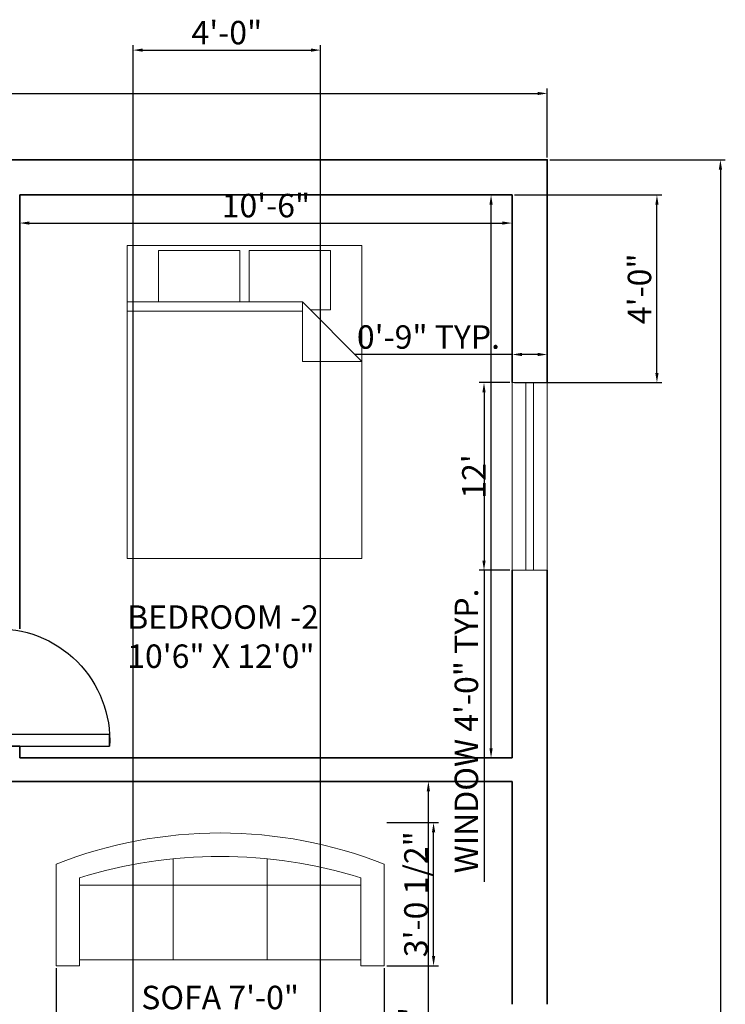
# Model space of a CAD drawing. Units: inches. Extents: x 2117 to 2588, y 1610 to 2201.
# Tile 4 of 4: x 2407 to 2588, y 1920 to 2172. Entities that reach past the tile are written whole.
import ezdxf

# ---------------------------------------------------------------- set-up
doc = ezdxf.new("R2010")
doc.units = ezdxf.units.IN
for name, color, linetype, lineweight in [('A-ANNO-DIMS', 2, 'Continuous', 18), ('A-AREA-IDEN', 7, 'Continuous', 25), ('A-DOOR', 4, 'Continuous', 25), ('A-FURN', 8, 'Continuous', 18), ('A-WALL', 7, 'Continuous', 35), ('WINDOW', 150, 'Continuous', 18)]:
    doc.layers.add(name, color=color, linetype=linetype, lineweight=lineweight)
doc.styles.get("Standard").update_dxf_attribs({"font": 'arial.ttf'})
doc.dimstyles.new('ISO-25', dxfattribs={"dimtxt": 6, "dimasz": 2.5, "dimexe": 1.25, "dimexo": 0.625, "dimtad": 1, "dimlunit": 3, "dimtxsty": 'Standard', "dimcen": 2.5, "dimadec": 0, "dimazin": 0, "dimtfac": 1, "dimtmove": 0, "dimatfit": 3, "dimfxl": 1, "dimarcsym": 0})

# ---------------------------------------------------------------- blocks, each defined once
blk = doc.blocks.new('*D1')
at = {"layer": 'A-ANNO-DIMS', "color": 0, "lineweight": -2, "transparency": 16777216}
for p, q in [((2407.08, 2126.4), (2407.08, 2118.59)), ((2533.08, 2126.4), (2533.08, 2118.59)), ((2409.58, 2119.84), (2530.58, 2119.84))]:
    blk.add_line(p, q, dxfattribs=at)
at = {"layer": 'A-ANNO-DIMS', "color": 0, "transparency": 16777216}
for points in [[(2409.58, 2120.26), (2409.58, 2119.43), (2407.08, 2119.84)], [(2530.58, 2120.26), (2530.58, 2119.43), (2533.08, 2119.84)]]:
    blk.add_solid(points, dxfattribs=at)
at = {"layer": 'Defpoints', "color": 0, "transparency": 16777216}
for p in [(2407.08, 2127.03), (2533.08, 2127.03), (2533.08, 2119.84)]:
    blk.add_point(p, dxfattribs=at)
at = {"layer": 'A-ANNO-DIMS', "color": 0, "transparency": 16777216, "insert": (2470.08, 2123.53), "char_height": 6, "attachment_point": 5}
blk.add_mtext('10\'-6"', dxfattribs=at)
blk = doc.blocks.new('*D2')
at = {"layer": 'A-ANNO-DIMS', "color": 0, "lineweight": -2, "transparency": 16777216}
for p, q in [((2532.45, 2127.03), (2526.43, 2127.03)), ((2527.68, 1985.53), (2527.68, 2124.53)), ((2532.45, 1983.03), (2526.43, 1983.03))]:
    blk.add_line(p, q, dxfattribs=at)
at = {"layer": 'A-ANNO-DIMS', "color": 0, "transparency": 16777216}
for points in [[(2527.27, 2124.53), (2528.1, 2124.53), (2527.68, 2127.03)], [(2527.27, 1985.53), (2528.1, 1985.53), (2527.68, 1983.03)]]:
    blk.add_solid(points, dxfattribs=at)
at = {"layer": 'Defpoints', "color": 0, "transparency": 16777216}
for p in [(2527.68, 2127.03), (2533.08, 2127.03), (2533.08, 1983.03)]:
    blk.add_point(p, dxfattribs=at)
at = {"layer": 'A-ANNO-DIMS', "color": 0, "transparency": 16777216, "insert": (2524.05, 2055.03), "char_height": 6, "attachment_point": 5, "rotation": 90}
blk.add_mtext("12'", dxfattribs=at)
blk = doc.blocks.new('*D16')
at = {"layer": 'A-ANNO-DIMS', "color": 0, "lineweight": -2, "transparency": 16777216}
for p, q in [((2532.45, 1977.03), (2510.4, 1977.03)), ((2511.65, 1841.53), (2511.65, 1974.53)), ((2532.45, 1839.03), (2510.4, 1839.03))]:
    blk.add_line(p, q, dxfattribs=at)
at = {"layer": 'A-ANNO-DIMS', "color": 0, "transparency": 16777216}
for points in [[(2511.23, 1974.53), (2512.06, 1974.53), (2511.65, 1977.03)], [(2511.23, 1841.53), (2512.06, 1841.53), (2511.65, 1839.03)]]:
    blk.add_solid(points, dxfattribs=at)
at = {"layer": 'Defpoints', "color": 0, "transparency": 16777216}
for p in [(2511.65, 1977.03), (2533.08, 1977.03), (2533.08, 1839.03)]:
    blk.add_point(p, dxfattribs=at)
at = {"layer": 'A-ANNO-DIMS', "color": 0, "transparency": 16777216, "insert": (2507.96, 1908.03), "char_height": 6, "attachment_point": 5, "rotation": 90}
blk.add_mtext('11\'-6"', dxfattribs=at)
blk = doc.blocks.new('Sofa - Roundback 7 ft.')
for p, q in [((-12.00002, -32.4421), (-12.00003, -6.5971)), ((11.99997, -32.4421), (11.99998, -6.5971)), ((-36.000027, -34), (-36.000027, -11.4696)), ((35.99998, -34), (35.99998, -11.4696)), ((-35.999844, -13.3819), (35.9998, -13.3819)), ((-36.000027, -32.4421), (35.99998, -32.4421))]:
    blk.add_line(p, q)
for points in [[(-36.000027, -34), (-42.000027, -34), (-42.000027, -8)], [(41.99998, -8), (41.99998, -34), (35.99998, -34)]]:
    blk.add_lwpolyline(points)
for centre, radius, start, end in [((0, -114.25), 114.25, 68.43141, 111.5686), ((-0.00001, -127.1968), 121.1968, 72.72033, 107.2797)]:
    blk.add_arc(centre, radius, start, end)
blk = doc.blocks.new('Bed - Queen')
for p, q in [((0, -80.00003), (0, 0)), ((0, 0), (59.99999, 0)), ((59.99999, 0), (59.99999, -80.00003)), ((7.99999, -1.2), (28.79998, -1.2)), ((7.99999, -14.4), (7.99999, -1.2)), ((28.79998, -1.2), (28.79998, -14.4)), ((31.19999, -1.2), (51.99999, -1.2)), ((31.19999, -14.4), (31.19999, -1.2)), ((51.99999, -1.2), (51.99999, -16.4)), ((0, -14.4), (44.8, -14.4)), ((59.99999, -29.6), (44.8, -14.4)), ((44.8, -14.4), (44.8, -29.6)), ((44.8, -16.8), (0, -16.8)), ((51.99999, -16.4), (46.79936, -16.4)), ((44.8, -29.6), (59.99999, -29.6)), ((59.99999, -80.00003), (0, -80.00003))]:
    blk.add_line(p, q)
blk = doc.blocks.new('*D30')
at = {"layer": 'A-ANNO-DIMS', "color": 0, "lineweight": -2, "transparency": 16777216}
for p, q in [((2158.08, 2136.65), (2158.08, 2154.24)), ((2542.08, 2136.65), (2542.08, 2154.24)), ((2160.58, 2152.99), (2539.58, 2152.99))]:
    blk.add_line(p, q, dxfattribs=at)
at = {"layer": 'A-ANNO-DIMS', "color": 0, "transparency": 16777216}
for points in [[(2160.58, 2153.4), (2160.58, 2152.57), (2158.08, 2152.99)], [(2539.58, 2153.4), (2539.58, 2152.57), (2542.08, 2152.99)]]:
    blk.add_solid(points, dxfattribs=at)
at = {"layer": 'Defpoints', "color": 0, "transparency": 16777216}
for p in [(2542.08, 2152.99), (2158.08, 2136.03), (2542.08, 2136.03)]:
    blk.add_point(p, dxfattribs=at)
at = {"layer": 'A-ANNO-DIMS', "color": 0, "transparency": 16777216, "insert": (2350.08, 2156.68), "char_height": 6, "attachment_point": 5}
blk.add_mtext("32'", dxfattribs=at)
blk = doc.blocks.new('*D31')
at = {"layer": 'A-ANNO-DIMS', "color": 0, "lineweight": -2, "transparency": 16777216}
for p, q in [((2542.7, 2136.03), (2587.62, 2136.03)), ((2586.37, 2133.53), (2586.37, 1658.53)), ((2542.7, 1656.03), (2587.62, 1656.03))]:
    blk.add_line(p, q, dxfattribs=at)
at = {"layer": 'A-ANNO-DIMS', "color": 0, "transparency": 16777216}
for points in [[(2585.96, 2133.53), (2586.79, 2133.53), (2586.37, 2136.03)], [(2585.96, 1658.53), (2586.79, 1658.53), (2586.37, 1656.03)]]:
    blk.add_solid(points, dxfattribs=at)
at = {"layer": 'Defpoints', "color": 0, "transparency": 16777216}
for p in [(2542.08, 2136.03), (2542.08, 1656.03), (2586.37, 1656.03)]:
    blk.add_point(p, dxfattribs=at)
at = {"layer": 'A-ANNO-DIMS', "color": 0, "transparency": 16777216, "insert": (2582.68, 1896.03), "char_height": 6, "attachment_point": 5, "rotation": 90}
blk.add_mtext("40'", dxfattribs=at)
blk = doc.blocks.new('WIN-48IN-9IN-WALL')
for p, q in [((9, 48), (0, 48)), ((0, 0), (0, 48)), ((3.5, 0), (3.5, 48)), ((5.5, 0), (5.5, 48)), ((9, 0), (9, 48)), ((9, 0), (0, 0))]:
    blk.add_line(p, q)
blk = doc.blocks.new('DOOR-SWING-30IN')
blk.add_lwpolyline([(30.04, 0), (0.04, 0), (0.04, 3), (30.04, 3)], close=True)
blk.add_arc((28.54, 1.5), 28.54, 86.9872, 183.0128)
blk = doc.blocks.new('*D37')
at = {"layer": 'A-ANNO-DIMS', "color": 0, "lineweight": -2, "transparency": 16777216}
for p, q in [((2532.45, 2079.03), (2524.63, 2079.03)), ((2525.88, 2076.53), (2525.88, 2033.53)), ((2532.45, 2031.03), (2524.63, 2031.03)), ((2525.88, 2031.03), (2525.88, 1951.35))]:
    blk.add_line(p, q, dxfattribs=at)
at = {"layer": 'A-ANNO-DIMS', "color": 0, "transparency": 16777216}
for points in [[(2525.46, 2076.53), (2526.29, 2076.53), (2525.88, 2079.03)], [(2525.46, 2033.53), (2526.29, 2033.53), (2525.88, 2031.03)]]:
    blk.add_solid(points, dxfattribs=at)
at = {"layer": 'Defpoints', "color": 0, "transparency": 16777216}
for p in [(2533.08, 2079.03), (2525.88, 2031.03), (2533.08, 2031.03)]:
    blk.add_point(p, dxfattribs=at)
at = {"layer": 'A-ANNO-DIMS', "color": 0, "transparency": 16777216, "insert": (2522.15, 1989.94), "char_height": 6, "attachment_point": 5, "rotation": 90}
blk.add_mtext('WINDOW 4\'-0" TYP.', dxfattribs=at)
blk = doc.blocks.new('*D38')
at = {"layer": 'A-ANNO-DIMS', "color": 0, "lineweight": -2, "transparency": 16777216}
for p, q in [((2533.08, 2086.23), (2492.75, 2086.23)), ((2533.08, 2079.65), (2533.08, 2087.48)), ((2539.58, 2086.23), (2535.58, 2086.23)), ((2542.08, 2079.65), (2542.08, 2087.48))]:
    blk.add_line(p, q, dxfattribs=at)
at = {"layer": 'A-ANNO-DIMS', "color": 0, "transparency": 16777216}
for points in [[(2535.58, 2086.65), (2535.58, 2085.81), (2533.08, 2086.23)], [(2539.58, 2086.65), (2539.58, 2085.81), (2542.08, 2086.23)]]:
    blk.add_solid(points, dxfattribs=at)
at = {"layer": 'Defpoints', "color": 0, "transparency": 16777216}
for p in [(2533.08, 2086.23), (2533.08, 2079.03), (2542.08, 2079.03)]:
    blk.add_point(p, dxfattribs=at)
at = {"layer": 'A-ANNO-DIMS', "color": 0, "transparency": 16777216, "insert": (2511.66, 2089.92), "char_height": 6, "attachment_point": 5}
blk.add_mtext('0\'-9" TYP.', dxfattribs=at)
blk = doc.blocks.new('*D47')
at = {"layer": 'A-ANNO-DIMS', "color": 0, "lineweight": -2, "transparency": 16777216}
for p, q in [((2403.45, 2120.46), (2403.45, 2156.7)), ((2399.12, 2120.46), (2404.7, 2120.46)), ((2403.45, 2089.91), (2403.45, 2117.96)), ((2399.12, 2087.41), (2404.7, 2087.41))]:
    blk.add_line(p, q, dxfattribs=at)
at = {"layer": 'A-ANNO-DIMS', "color": 0, "transparency": 16777216}
for points in [[(2403.04, 2117.96), (2403.87, 2117.96), (2403.45, 2120.46)], [(2403.04, 2089.91), (2403.87, 2089.91), (2403.45, 2087.41)]]:
    blk.add_solid(points, dxfattribs=at)
at = {"layer": 'Defpoints', "color": 0, "transparency": 16777216}
for p in [(2398.5, 2120.46), (2403.45, 2120.46), (2398.5, 2087.41)]:
    blk.add_point(p, dxfattribs=at)
at = {"layer": 'A-ANNO-DIMS', "color": 0, "transparency": 16777216, "insert": (2399.73, 2139.83), "char_height": 6, "attachment_point": 5, "rotation": 90}
blk.add_mtext('WC 2\'-9"', dxfattribs=at)
blk = doc.blocks.new('*D49')
at = {"layer": 'A-ANNO-DIMS', "color": 0, "lineweight": -2, "transparency": 16777216}
for p, q in [((2416.37, 1929.23), (2416.37, 1916.01)), ((2500.37, 1929.23), (2500.37, 1916.01)), ((2418.87, 1917.26), (2497.87, 1917.26))]:
    blk.add_line(p, q, dxfattribs=at)
at = {"layer": 'A-ANNO-DIMS', "color": 0, "transparency": 16777216}
for points in [[(2418.87, 1917.67), (2418.87, 1916.84), (2416.37, 1917.26)], [(2497.87, 1917.67), (2497.87, 1916.84), (2500.37, 1917.26)]]:
    blk.add_solid(points, dxfattribs=at)
at = {"layer": 'Defpoints', "color": 0, "transparency": 16777216}
for p in [(2416.37, 1929.86), (2500.37, 1929.86), (2500.37, 1917.26)]:
    blk.add_point(p, dxfattribs=at)
at = {"layer": 'A-ANNO-DIMS', "color": 0, "transparency": 16777216, "insert": (2458.37, 1920.99), "char_height": 6, "attachment_point": 5}
blk.add_mtext('SOFA 7\'-0"', dxfattribs=at)
blk = doc.blocks.new('*D50')
at = {"layer": 'A-ANNO-DIMS', "color": 0, "lineweight": -2, "transparency": 16777216}
for p, q in [((2501, 1966.52), (2514.22, 1966.52)), ((2512.97, 1932.36), (2512.97, 1964.02)), ((2501, 1929.86), (2514.22, 1929.86))]:
    blk.add_line(p, q, dxfattribs=at)
at = {"layer": 'A-ANNO-DIMS', "color": 0, "transparency": 16777216}
for points in [[(2512.56, 1964.02), (2513.39, 1964.02), (2512.97, 1966.52)], [(2512.56, 1932.36), (2513.39, 1932.36), (2512.97, 1929.86)]]:
    blk.add_solid(points, dxfattribs=at)
at = {"layer": 'Defpoints', "color": 0, "transparency": 16777216}
for p in [(2500.37, 1966.52), (2512.97, 1966.52), (2500.37, 1929.86)]:
    blk.add_point(p, dxfattribs=at)
at = {"layer": 'A-ANNO-DIMS', "color": 0, "transparency": 16777216, "insert": (2509.24, 1948.19), "char_height": 6, "attachment_point": 5, "rotation": 90}
blk.add_mtext('3\'-0 1/2"', dxfattribs=at)
blk = doc.blocks.new('*D65')
at = {"layer": 'A-ANNO-DIMS', "color": 0, "lineweight": -2, "transparency": 16777216}
for p, q in [((2533.7, 2127.03), (2571.38, 2127.03)), ((2570.13, 2081.53), (2570.13, 2124.53)), ((2533.7, 2079.03), (2571.38, 2079.03))]:
    blk.add_line(p, q, dxfattribs=at)
at = {"layer": 'A-ANNO-DIMS', "color": 0, "transparency": 16777216}
for points in [[(2569.71, 2124.53), (2570.54, 2124.53), (2570.13, 2127.03)], [(2569.71, 2081.53), (2570.54, 2081.53), (2570.13, 2079.03)]]:
    blk.add_solid(points, dxfattribs=at)
at = {"layer": 'Defpoints', "color": 0, "transparency": 16777216}
for p in [(2533.08, 2127.03), (2570.13, 2127.03), (2533.08, 2079.03)]:
    blk.add_point(p, dxfattribs=at)
at = {"layer": 'A-ANNO-DIMS', "color": 0, "transparency": 16777216, "insert": (2566.44, 2103.03), "char_height": 6, "attachment_point": 5, "rotation": 90}
blk.add_mtext('4\'-0"', dxfattribs=at)
blk = doc.blocks.new('*D75')
at = {"layer": 'A-ANNO-DIMS', "color": 0, "lineweight": -2, "transparency": 16777216}
for p, q in [((2436.08, 1833.65), (2436.08, 2165.33)), ((2438.58, 2164.08), (2481.58, 2164.08)), ((2484.08, 1833.65), (2484.08, 2165.33))]:
    blk.add_line(p, q, dxfattribs=at)
at = {"layer": 'A-ANNO-DIMS', "color": 0, "transparency": 16777216}
for points in [[(2438.58, 2164.5), (2438.58, 2163.66), (2436.08, 2164.08)], [(2481.58, 2164.5), (2481.58, 2163.66), (2484.08, 2164.08)]]:
    blk.add_solid(points, dxfattribs=at)
at = {"layer": 'Defpoints', "color": 0, "transparency": 16777216}
for p in [(2484.08, 2164.08), (2436.08, 1833.03), (2484.08, 1833.03)]:
    blk.add_point(p, dxfattribs=at)
at = {"layer": 'A-ANNO-DIMS', "color": 0, "transparency": 16777216, "insert": (2460.08, 2167.77), "char_height": 6, "attachment_point": 5}
blk.add_mtext('4\'-0"', dxfattribs=at)

msp = doc.modelspace()

# ---------------------------------------------------------------- linework, layer by layer
at = {"layer": 'A-WALL'}
for p, q in [((2407.076, 2127.029), (2533.076, 2127.029)), ((2407.076, 2016.029), (2407.076, 2127.029)), ((2533.076, 2127.029), (2533.076, 2079.029)), ((2533.076, 2031.029), (2533.076, 1983.029)), ((2407.076, 1986.029), (2400.076, 1986.029)), ((2407.076, 1983.029), (2407.076, 1986.029)), ((2407.076, 1983.029), (2533.076, 1983.029)), ((2400.076, 1977.029), (2533.076, 1977.029)), ((2533.076, 1977.029), (2533.076, 1920.029))]:
    msp.add_line(p, q, dxfattribs=at)
for points in [[(2385.076, 2136.029), (2542.076, 2136.029), (2542.076, 2079.029)], [(2542.076, 2031.029), (2542.076, 1920.029)]]:
    msp.add_lwpolyline(points, dxfattribs=at)

# ---------------------------------------------------------------- block references
at = {"layer": 'A-DOOR', "extrusion": (0, 0, -1), "zscale": -1}
msp.add_blockref('DOOR-SWING-30IN', (-2430.116, 1986.029), dxfattribs=at)
at = {"layer": 'A-FURN'}
for name, p in [('Bed - Queen', (2434.598, 2114.066)), ('Sofa - Roundback 7 ft.', (2458.372, 1963.856))]:
    msp.add_blockref(name, p, dxfattribs=at)
at = {"layer": 'WINDOW', "rotation": 180}
msp.add_blockref('WIN-48IN-9IN-WALL', (2542.076, 2079.028), dxfattribs=at)

# ---------------------------------------------------------------- texts
at = {"layer": 'A-AREA-IDEN', "insert": (2434.598, 2022.064), "char_height": 6, "attachment_point": 1}
msp.add_mtext_dynamic_manual_height_columns('{\\fArial|b1|i0|c0|p34;BEDROOM -2 \\P10\'6" X 12\'0"}', width=67.92239, gutter_width=12.5, heights=[0], dxfattribs=at)

# ---------------------------------------------------------------- dimensions: what is measured, and where the dimension line sits
at = {"layer": 'A-ANNO-DIMS'}
for base, p1, p2, override, picture, middle in [((2484.076, 2164.079), (2436.076, 1833.029), (2484.076, 1833.029), {"dimdec": 1, "dimlfac": 1, "dimrnd": 0, "dimzin": 1, "dimdsep": 46, "dimlunit": 4, "dimfrac": 2}, '*D75', (2460.076, 2167.767)), ((2542.076, 2152.986), (2158.076, 2136.029), (2542.076, 2136.029), {"dimclrd": 0, "dimclre": 0, "dimclrt": 0}, '*D30', (2350.076, 2156.677)), ((2533.076, 2119.844), (2407.076, 2127.029), (2533.076, 2127.029), {"dimclrd": 0, "dimclre": 0, "dimclrt": 0}, '*D1', (2470.076, 2123.532))]:
    dim = msp.add_linear_dim(base=base, p1=p1, p2=p2, dimstyle='ISO-25', override=override, dxfattribs=at)
    dim.commit()
    dim.dimension.update_dxf_attribs({"geometry": picture, "text_midpoint": middle})
for base, p1, p2, angle, text, picture, middle in [((2403.454, 2120.458), (2398.497, 2087.412), (2398.497, 2120.458), 90, 'WC <>', '*D47', (2399.726, 2139.827)), ((2533.076, 2086.229), (2542.076, 2079.029), (2533.076, 2079.029), 180, '<> TYP.', '*D38', (2511.664, 2089.917)), ((2525.876, 2031.029), (2533.076, 2079.029), (2533.076, 2031.029), 270, 'WINDOW <> TYP.', '*D37', (2522.147, 1989.941))]:
    dim = msp.add_linear_dim(base=base, p1=p1, p2=p2, angle=angle, text=text, dimstyle='ISO-25', override={"dimdec": 1, "dimlfac": 1, "dimrnd": 0, "dimzin": 1, "dimdsep": 46, "dimlunit": 4, "dimfrac": 2}, dxfattribs=at)
    dim.commit()
    dim.dimension.update_dxf_attribs({"geometry": picture, "text_midpoint": middle})
for base, p1, p2, override, picture, middle in [((2586.372, 1656.029), (2542.076, 2136.029), (2542.076, 1656.029), {"dimclrd": 0, "dimclre": 0, "dimclrt": 0}, '*D31', (2582.684, 1896.029)), ((2527.685, 2127.029), (2533.076, 1983.029), (2533.076, 2127.029), {"dimclrd": 0, "dimclre": 0, "dimclrt": 0}, '*D2', (2524.048, 2055.029)), ((2570.126, 2127.029), (2533.076, 2079.029), (2533.076, 2127.029), {"dimdec": 1, "dimlfac": 1, "dimrnd": 0, "dimzin": 1, "dimdsep": 46, "dimlunit": 4, "dimfrac": 2}, '*D65', (2566.437, 2103.029)), ((2511.647, 1977.029), (2533.076, 1839.029), (2533.076, 1977.029), {"dimclrd": 0, "dimclre": 0, "dimclrt": 0}, '*D16', (2507.958, 1908.029)), ((2512.972, 1966.523), (2500.372, 1929.856), (2500.372, 1966.523), {"dimdec": 1, "dimlfac": 1, "dimrnd": 0, "dimzin": 1, "dimdsep": 46, "dimlunit": 4, "dimfrac": 2}, '*D50', (2509.243, 1948.19))]:
    dim = msp.add_linear_dim(base=base, p1=p1, p2=p2, angle=90, dimstyle='ISO-25', override=override, dxfattribs=at)
    dim.commit()
    dim.dimension.update_dxf_attribs({"geometry": picture, "text_midpoint": middle})
dim = msp.add_linear_dim(base=(2500.372, 1917.256), p1=(2416.372, 1929.856), p2=(2500.372, 1929.856), text='SOFA <>', dimstyle='ISO-25', override={"dimdec": 1, "dimlfac": 1, "dimrnd": 0, "dimzin": 1, "dimdsep": 46, "dimlunit": 4, "dimfrac": 2}, dxfattribs=at)
dim.commit()
dim.dimension.update_dxf_attribs({"geometry": '*D49', "text_midpoint": (2458.372, 1920.986)})

doc.saveas('drawing.dxf')
